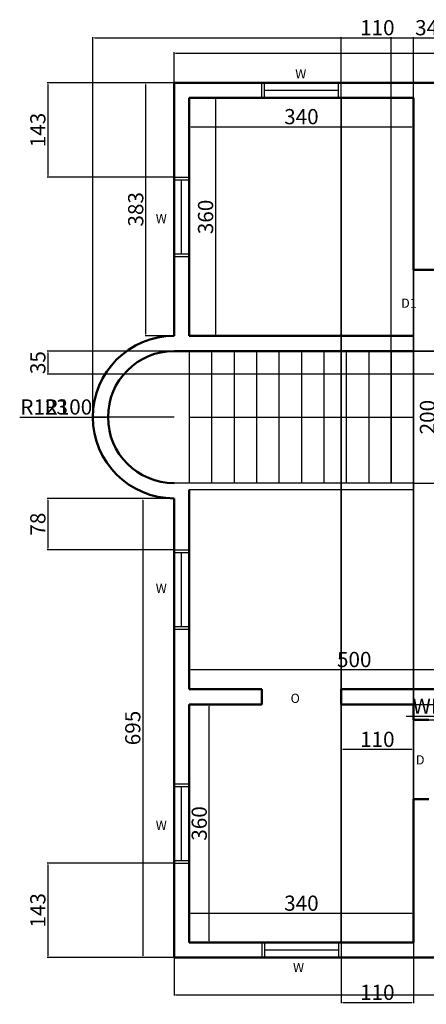
# Model space of a CAD drawing. Units: centimetres. Extents: x 6294 to 7898, y 3240 to 4730.
# Tile 1 of 3: x 6294 to 6910, y 3240 to 4730. Entities that reach past the tile are written whole.
import ezdxf

# ---------------------------------------------------------------- set-up
doc = ezdxf.new("R2010")
doc.units = ezdxf.units.CM
for name, color, linetype, lineweight in [('A-ANNO-DIMS', 2, 'Continuous', 18), ('A-ANNO-TEXT', 7, 'Continuous', 25), ('A-FLOR-STRS', 3, 'Continuous', 25), ('A-GLAZ', 4, 'Continuous', 25), ('A-WALL', 7, 'Continuous', 50)]:
    doc.layers.add(name, color=color, linetype=linetype, lineweight=lineweight)
doc.styles.get("Standard").update_dxf_attribs({"font": 'arial.ttf'})
doc.dimstyles.new('ISO-25', dxfattribs={"dimtxt": 23, "dimasz": 2.5, "dimexe": 1.25, "dimexo": 0.625, "dimtad": 1, "dimtxsty": 'Standard', "dimcen": 2.5, "dimadec": 0, "dimazin": 0, "dimtfac": 1, "dimtmove": 0, "dimatfit": 3, "dimfxl": 1, "dimarcsym": 0})

# ---------------------------------------------------------------- blocks, each defined once
blk = doc.blocks.new('*D2')
at = {"layer": 'A-ANNO-DIMS', "color": 0, "lineweight": -2, "transparency": 16777216}
for p, q in [((6551.4, 4611.8), (6592.1, 4611.8)), ((6590.8, 4254.3), (6590.8, 4609.3)), ((6551.4, 4251.8), (6592.1, 4251.8))]:
    blk.add_line(p, q, dxfattribs=at)
at = {"layer": 'A-ANNO-DIMS', "color": 0, "transparency": 16777216}
for points in [[(6590.4, 4609.3), (6591.3, 4609.3), (6590.8, 4611.8)], [(6590.4, 4254.3), (6591.3, 4254.3), (6590.8, 4251.8)]]:
    blk.add_solid(points, dxfattribs=at)
at = {"layer": 'Defpoints', "color": 0, "transparency": 16777216}
for p in [(6550.7, 4611.8), (6590.8, 4611.8), (6550.7, 4251.8)]:
    blk.add_point(p, dxfattribs=at)
at = {"layer": 'A-ANNO-DIMS', "color": 0, "transparency": 16777216, "insert": (6578.5, 4431.8), "char_height": 23, "attachment_point": 5, "rotation": 90}
blk.add_mtext('360', dxfattribs=at)
blk = doc.blocks.new('*D3')
at = {"layer": 'A-ANNO-DIMS', "color": 0, "lineweight": -2, "transparency": 16777216}
for p, q in [((6550.7, 4611.2), (6550.7, 4566.9)), ((6890.7, 4611.2), (6890.7, 4566.9)), ((6553.2, 4568.2), (6888.2, 4568.2))]:
    blk.add_line(p, q, dxfattribs=at)
at = {"layer": 'A-ANNO-DIMS', "color": 0, "transparency": 16777216}
for points in [[(6553.2, 4568.6), (6553.2, 4567.8), (6550.7, 4568.2)], [(6888.2, 4568.6), (6888.2, 4567.8), (6890.7, 4568.2)]]:
    blk.add_solid(points, dxfattribs=at)
at = {"layer": 'Defpoints', "color": 0, "transparency": 16777216}
for p in [(6550.7, 4611.8), (6890.7, 4611.8), (6890.7, 4568.2)]:
    blk.add_point(p, dxfattribs=at)
at = {"layer": 'A-ANNO-DIMS', "color": 0, "transparency": 16777216, "insert": (6720.7, 4580.6), "char_height": 23, "attachment_point": 5}
blk.add_mtext('340', dxfattribs=at)
blk = doc.blocks.new('*D18')
at = {"layer": 'A-ANNO-DIMS', "color": 0, "lineweight": -2, "transparency": 16777216}
for p, q in [((6551.4, 3693.8), (6582.5, 3693.8)), ((6581.2, 3336.3), (6581.2, 3691.3)), ((6551.4, 3333.8), (6582.5, 3333.8))]:
    blk.add_line(p, q, dxfattribs=at)
at = {"layer": 'A-ANNO-DIMS', "color": 0, "transparency": 16777216}
for points in [[(6580.8, 3691.3), (6581.7, 3691.3), (6581.2, 3693.8)], [(6580.8, 3336.3), (6581.7, 3336.3), (6581.2, 3333.8)]]:
    blk.add_solid(points, dxfattribs=at)
at = {"layer": 'Defpoints', "color": 0, "transparency": 16777216}
for p in [(6550.7, 3693.8), (6581.2, 3693.8), (6550.7, 3333.8)]:
    blk.add_point(p, dxfattribs=at)
at = {"layer": 'A-ANNO-DIMS', "color": 0, "transparency": 16777216, "insert": (6568.9, 3513.8), "char_height": 23, "attachment_point": 5, "rotation": 90}
blk.add_mtext('360', dxfattribs=at)
blk = doc.blocks.new('*D19')
at = {"layer": 'A-ANNO-DIMS', "color": 0, "lineweight": -2, "transparency": 16777216}
for p, q in [((6550.7, 3334.5), (6550.7, 3379.1)), ((6553.2, 3377.9), (6888.2, 3377.9)), ((6890.7, 3334.5), (6890.7, 3379.1))]:
    blk.add_line(p, q, dxfattribs=at)
at = {"layer": 'A-ANNO-DIMS', "color": 0, "transparency": 16777216}
for points in [[(6553.2, 3378.3), (6553.2, 3377.4), (6550.7, 3377.9)], [(6888.2, 3378.3), (6888.2, 3377.4), (6890.7, 3377.9)]]:
    blk.add_solid(points, dxfattribs=at)
at = {"layer": 'Defpoints', "color": 0, "transparency": 16777216}
for p in [(6890.7, 3377.9), (6550.7, 3333.8), (6890.7, 3333.8)]:
    blk.add_point(p, dxfattribs=at)
at = {"layer": 'A-ANNO-DIMS', "color": 0, "transparency": 16777216, "insert": (6720.7, 3390.2), "char_height": 23, "attachment_point": 5}
blk.add_mtext('340', dxfattribs=at)
blk = doc.blocks.new('*D20')
at = {"layer": 'A-ANNO-DIMS', "color": 0, "lineweight": -2, "transparency": 16777216}
for p, q in [((6550.7, 3717.5), (6550.7, 3747.9)), ((6553.2, 3746.6), (7048.2, 3746.6)), ((7050.7, 3717.5), (7050.7, 3747.9))]:
    blk.add_line(p, q, dxfattribs=at)
at = {"layer": 'A-ANNO-DIMS', "color": 0, "transparency": 16777216}
for points in [[(6553.2, 3747), (6553.2, 3746.2), (6550.7, 3746.6)], [(7048.2, 3747), (7048.2, 3746.2), (7050.7, 3746.6)]]:
    blk.add_solid(points, dxfattribs=at)
at = {"layer": 'Defpoints', "color": 0, "transparency": 16777216}
for p in [(7050.7, 3746.6), (6550.7, 3716.8), (7050.7, 3716.8)]:
    blk.add_point(p, dxfattribs=at)
at = {"layer": 'A-ANNO-DIMS', "color": 0, "transparency": 16777216, "insert": (6800.7, 3759), "char_height": 23, "attachment_point": 5}
blk.add_mtext('500', dxfattribs=at)
blk = doc.blocks.new('*D22')
at = {"layer": 'A-ANNO-DIMS', "color": 0, "lineweight": -2, "transparency": 16777216}
for p, q in [((6891.4, 4228.8), (6928.2, 4228.8)), ((6926.9, 4226.3), (6926.9, 4031.3)), ((6891.4, 4028.8), (6928.2, 4028.8))]:
    blk.add_line(p, q, dxfattribs=at)
at = {"layer": 'A-ANNO-DIMS', "color": 0, "transparency": 16777216}
for points in [[(6926.5, 4226.3), (6927.3, 4226.3), (6926.9, 4228.8)], [(6926.5, 4031.3), (6927.3, 4031.3), (6926.9, 4028.8)]]:
    blk.add_solid(points, dxfattribs=at)
at = {"layer": 'Defpoints', "color": 0, "transparency": 16777216}
for p in [(6890.7, 4228.8), (6890.7, 4028.8), (6926.9, 4028.8)]:
    blk.add_point(p, dxfattribs=at)
at = {"layer": 'A-ANNO-DIMS', "color": 0, "transparency": 16777216, "insert": (6914.6, 4128.8), "char_height": 23, "attachment_point": 5, "rotation": 90}
blk.add_mtext('200', dxfattribs=at)
blk = doc.blocks.new('*D23')
at = {"layer": 'A-ANNO-DIMS', "color": 0, "lineweight": -2, "transparency": 16777216}
for p, q in [((6527.7, 4635.5), (6527.7, 4681.1)), ((6530.2, 4679.8), (7596.2, 4679.8)), ((7598.7, 4635.5), (7598.7, 4681.1))]:
    blk.add_line(p, q, dxfattribs=at)
at = {"layer": 'A-ANNO-DIMS', "color": 0, "transparency": 16777216}
for points in [[(6530.2, 4680.2), (6530.2, 4679.4), (6527.7, 4679.8)], [(7596.2, 4680.2), (7596.2, 4679.4), (7598.7, 4679.8)]]:
    blk.add_solid(points, dxfattribs=at)
at = {"layer": 'Defpoints', "color": 0, "transparency": 16777216}
for p in [(7598.7, 4679.8), (6527.7, 4634.8), (7598.7, 4634.8)]:
    blk.add_point(p, dxfattribs=at)
at = {"layer": 'A-ANNO-DIMS', "color": 0, "transparency": 16777216, "insert": (7063.2, 4692.2), "char_height": 23, "attachment_point": 5}
blk.add_mtext('1071', dxfattribs=at)
blk = doc.blocks.new('*D26')
at = {"layer": 'A-ANNO-DIMS', "color": 0, "lineweight": -2, "transparency": 16777216}
for p, q in [((6527.7, 3310.2), (6527.7, 3253.3)), ((7396.7, 3310.2), (7396.7, 3253.3)), ((6530.2, 3254.6), (7394.2, 3254.6))]:
    blk.add_line(p, q, dxfattribs=at)
at = {"layer": 'A-ANNO-DIMS', "color": 0, "transparency": 16777216}
for points in [[(6530.2, 3255), (6530.2, 3254.2), (6527.7, 3254.6)], [(7394.2, 3255), (7394.2, 3254.2), (7396.7, 3254.6)]]:
    blk.add_solid(points, dxfattribs=at)
at = {"layer": 'Defpoints', "color": 0, "transparency": 16777216}
for p in [(6527.7, 3310.8), (7396.7, 3310.8), (7396.7, 3254.6)]:
    blk.add_point(p, dxfattribs=at)
at = {"layer": 'A-ANNO-DIMS', "color": 0, "transparency": 16777216, "insert": (6962.2, 3266.9), "char_height": 23, "attachment_point": 5}
blk.add_mtext('869', dxfattribs=at)
blk = doc.blocks.new('*D27')
at = {"layer": 'A-ANNO-DIMS', "color": 0, "lineweight": -2, "transparency": 16777216}
for p, q in [((6527.1, 4005.8), (6479.3, 4005.8)), ((6480.6, 4003.3), (6480.6, 3313.3)), ((6527.1, 3310.8), (6479.3, 3310.8))]:
    blk.add_line(p, q, dxfattribs=at)
at = {"layer": 'A-ANNO-DIMS', "color": 0, "transparency": 16777216}
for points in [[(6480.2, 4003.3), (6481, 4003.3), (6480.6, 4005.8)], [(6480.2, 3313.3), (6481, 3313.3), (6480.6, 3310.8)]]:
    blk.add_solid(points, dxfattribs=at)
at = {"layer": 'Defpoints', "color": 0, "transparency": 16777216}
for p in [(6527.7, 4005.8), (6480.6, 3310.8), (6527.7, 3310.8)]:
    blk.add_point(p, dxfattribs=at)
at = {"layer": 'A-ANNO-DIMS', "color": 0, "transparency": 16777216, "insert": (6468.2, 3658.3), "char_height": 23, "attachment_point": 5, "rotation": 90}
blk.add_mtext('695', dxfattribs=at)
blk = doc.blocks.new('*D28')
at = {"layer": 'A-ANNO-DIMS', "color": 0, "lineweight": -2, "transparency": 16777216}
for p, q in [((6527.1, 4634.8), (6483.8, 4634.8)), ((6485.1, 4254.3), (6485.1, 4632.3)), ((6527.1, 4251.8), (6483.8, 4251.8))]:
    blk.add_line(p, q, dxfattribs=at)
at = {"layer": 'A-ANNO-DIMS', "color": 0, "transparency": 16777216}
for points in [[(6484.7, 4632.3), (6485.5, 4632.3), (6485.1, 4634.8)], [(6484.7, 4254.3), (6485.5, 4254.3), (6485.1, 4251.8)]]:
    blk.add_solid(points, dxfattribs=at)
at = {"layer": 'Defpoints', "color": 0, "transparency": 16777216}
for p in [(6485.1, 4634.8), (6527.7, 4634.8), (6527.7, 4251.8)]:
    blk.add_point(p, dxfattribs=at)
at = {"layer": 'A-ANNO-DIMS', "color": 0, "transparency": 16777216, "insert": (6472.7, 4443.3), "char_height": 23, "attachment_point": 5, "rotation": 90}
blk.add_mtext('383', dxfattribs=at)
blk = doc.blocks.new('WIN-W-120CM')
for p, q in [((0, 23), (0, 0)), ((4, 23), (4, 0)), ((116, 23), (116, 0)), ((120, 23), (120, 0)), ((4, 11.5), (116, 11.5))]:
    blk.add_line(p, q)
blk = doc.blocks.new('*D32')
at = {"layer": 'A-ANNO-DIMS', "color": 0, "lineweight": -2, "transparency": 16777216}
for p, q in [((7163.7, 3693.2), (7163.7, 3674.6)), ((7283.7, 3693.2), (7283.7, 3674.6)), ((7163.7, 3675.8), (6879.3, 3675.8)), ((7281.2, 3675.8), (7166.2, 3675.8))]:
    blk.add_line(p, q, dxfattribs=at)
at = {"layer": 'A-ANNO-DIMS', "color": 0, "transparency": 16777216}
for points in [[(7166.2, 3676.3), (7166.2, 3675.4), (7163.7, 3675.8)], [(7281.2, 3676.3), (7281.2, 3675.4), (7283.7, 3675.8)]]:
    blk.add_solid(points, dxfattribs=at)
at = {"layer": 'Defpoints', "color": 0, "transparency": 16777216}
for p in [(7163.7, 3693.8), (7283.7, 3693.8), (7163.7, 3675.8)]:
    blk.add_point(p, dxfattribs=at)
at = {"layer": 'A-ANNO-DIMS', "color": 0, "transparency": 16777216, "insert": (7020.3, 3688.4), "char_height": 23, "attachment_point": 5}
blk.add_mtext('WINDOW 120 TYP.', dxfattribs=at)
blk = doc.blocks.new('*D39')
at = {"layer": 'A-ANNO-DIMS', "color": 0, "lineweight": -2, "transparency": 16777216}
for p, q in [((6404.7, 4129.5), (6404.7, 4704.1)), ((6407.2, 4702.8), (7596.2, 4702.8)), ((7598.7, 4635.5), (7598.7, 4704.1))]:
    blk.add_line(p, q, dxfattribs=at)
at = {"layer": 'A-ANNO-DIMS', "color": 0, "transparency": 16777216}
for points in [[(6407.2, 4703.3), (6407.2, 4702.4), (6404.7, 4702.8)], [(7596.2, 4703.3), (7596.2, 4702.4), (7598.7, 4702.8)]]:
    blk.add_solid(points, dxfattribs=at)
at = {"layer": 'Defpoints', "color": 0, "transparency": 16777216}
for p in [(7598.7, 4702.8), (7598.7, 4634.8), (6404.7, 4128.8)]:
    blk.add_point(p, dxfattribs=at)
at = {"layer": 'A-ANNO-DIMS', "color": 0, "transparency": 16777216, "insert": (7001.7, 4715.2), "char_height": 23, "attachment_point": 5}
blk.add_mtext('1194', dxfattribs=at)
blk = doc.blocks.new('*D40')
at = {"layer": 'A-ANNO-DIMS', "color": 0, "lineweight": -2, "transparency": 16777216}
for p, q in [((6856.7, 4029.5), (6856.7, 4704.1)), ((6859.2, 4702.8), (6888.2, 4702.8)), ((6890.7, 4029.5), (6890.7, 4704.1)), ((6890.7, 4702.8), (6927.3, 4702.8))]:
    blk.add_line(p, q, dxfattribs=at)
at = {"layer": 'A-ANNO-DIMS', "color": 0, "transparency": 16777216}
for points in [[(6859.2, 4703.3), (6859.2, 4702.4), (6856.7, 4702.8)], [(6888.2, 4703.3), (6888.2, 4702.4), (6890.7, 4702.8)]]:
    blk.add_solid(points, dxfattribs=at)
at = {"layer": 'Defpoints', "color": 0, "transparency": 16777216}
for p in [(6890.7, 4702.8), (6856.7, 4028.8), (6890.7, 4028.8)]:
    blk.add_point(p, dxfattribs=at)
at = {"layer": 'A-ANNO-DIMS', "color": 0, "transparency": 16777216, "insert": (6910.3, 4715.2), "char_height": 23, "attachment_point": 5}
blk.add_mtext('34', dxfattribs=at)
blk = doc.blocks.new('*D41')
at = {"layer": 'A-ANNO-DIMS', "color": 0, "lineweight": -2, "transparency": 16777216}
for p, q in [((6527.1, 4005.8), (6335.5, 4005.8)), ((6336.7, 4003.3), (6336.7, 3930.3)), ((6527.1, 3927.8), (6335.5, 3927.8))]:
    blk.add_line(p, q, dxfattribs=at)
at = {"layer": 'A-ANNO-DIMS', "color": 0, "transparency": 16777216}
for points in [[(6336.3, 4003.3), (6337.2, 4003.3), (6336.7, 4005.8)], [(6336.3, 3930.3), (6337.2, 3930.3), (6336.7, 3927.8)]]:
    blk.add_solid(points, dxfattribs=at)
at = {"layer": 'Defpoints', "color": 0, "transparency": 16777216}
for p in [(6527.7, 4005.8), (6336.7, 3927.8), (6527.7, 3927.8)]:
    blk.add_point(p, dxfattribs=at)
at = {"layer": 'A-ANNO-DIMS', "color": 0, "transparency": 16777216, "insert": (6324.4, 3966.8), "char_height": 23, "attachment_point": 5, "rotation": 90}
blk.add_mtext('78', dxfattribs=at)
blk = doc.blocks.new('*D42')
at = {"layer": 'A-ANNO-DIMS', "color": 0, "lineweight": -2, "transparency": 16777216}
for p, q in [((6780.7, 3334.5), (6780.7, 4704.1)), ((6783.2, 4702.8), (6888.2, 4702.8)), ((6890.7, 3334.5), (6890.7, 4704.1))]:
    blk.add_line(p, q, dxfattribs=at)
at = {"layer": 'A-ANNO-DIMS', "color": 0, "transparency": 16777216}
for points in [[(6783.2, 4703.3), (6783.2, 4702.4), (6780.7, 4702.8)], [(6888.2, 4703.3), (6888.2, 4702.4), (6890.7, 4702.8)]]:
    blk.add_solid(points, dxfattribs=at)
at = {"layer": 'Defpoints', "color": 0, "transparency": 16777216}
for p in [(6890.7, 4702.8), (6780.7, 3333.8), (6890.7, 3333.8)]:
    blk.add_point(p, dxfattribs=at)
at = {"layer": 'A-ANNO-DIMS', "color": 0, "transparency": 16777216, "insert": (6835.7, 4715.2), "char_height": 23, "attachment_point": 5}
blk.add_mtext('110', dxfattribs=at)
blk = doc.blocks.new('*D43')
at = {"layer": 'A-ANNO-DIMS', "color": 0, "lineweight": -2, "transparency": 16777216}
for p, q in [((6527.1, 3453.8), (6335.5, 3453.8)), ((6336.7, 3451.3), (6336.7, 3313.3)), ((6527.1, 3310.8), (6335.5, 3310.8))]:
    blk.add_line(p, q, dxfattribs=at)
at = {"layer": 'A-ANNO-DIMS', "color": 0, "transparency": 16777216}
for points in [[(6336.3, 3451.3), (6337.2, 3451.3), (6336.7, 3453.8)], [(6336.3, 3313.3), (6337.2, 3313.3), (6336.7, 3310.8)]]:
    blk.add_solid(points, dxfattribs=at)
at = {"layer": 'Defpoints', "color": 0, "transparency": 16777216}
for p in [(6527.7, 3453.8), (6336.7, 3310.8), (6527.7, 3310.8)]:
    blk.add_point(p, dxfattribs=at)
at = {"layer": 'A-ANNO-DIMS', "color": 0, "transparency": 16777216, "insert": (6324.4, 3382.3), "char_height": 23, "attachment_point": 5, "rotation": 90}
blk.add_mtext('143', dxfattribs=at)
blk = doc.blocks.new('*D44')
at = {"layer": 'A-ANNO-DIMS', "color": 0, "lineweight": -2, "transparency": 16777216}
for p, q in [((6891.4, 3693.8), (7668, 3693.8)), ((7666.7, 3691.3), (7666.7, 3673.3)), ((6891.4, 3670.8), (7668, 3670.8)), ((7666.7, 3670.8), (7666.7, 3633.8))]:
    blk.add_line(p, q, dxfattribs=at)
at = {"layer": 'A-ANNO-DIMS', "color": 0, "transparency": 16777216}
for points in [[(7666.3, 3691.3), (7667.2, 3691.3), (7666.7, 3693.8)], [(7666.3, 3673.3), (7667.2, 3673.3), (7666.7, 3670.8)]]:
    blk.add_solid(points, dxfattribs=at)
at = {"layer": 'Defpoints', "color": 0, "transparency": 16777216}
for p in [(6890.7, 3693.8), (6890.7, 3670.8), (7666.7, 3670.8)]:
    blk.add_point(p, dxfattribs=at)
at = {"layer": 'A-ANNO-DIMS', "color": 0, "transparency": 16777216, "insert": (7654.4, 3651.1), "char_height": 23, "attachment_point": 5, "rotation": 90}
blk.add_mtext('23', dxfattribs=at)
blk = doc.blocks.new('*D45')
at = {"layer": 'A-ANNO-DIMS', "color": 0, "lineweight": -2, "transparency": 16777216}
for p, q in [((6780.7, 4611.2), (6780.7, 3241.6)), ((6890.7, 4611.2), (6890.7, 3241.6)), ((6783.2, 3242.8), (6888.2, 3242.8))]:
    blk.add_line(p, q, dxfattribs=at)
at = {"layer": 'A-ANNO-DIMS', "color": 0, "transparency": 16777216}
for points in [[(6783.2, 3243.3), (6783.2, 3242.4), (6780.7, 3242.8)], [(6888.2, 3243.3), (6888.2, 3242.4), (6890.7, 3242.8)]]:
    blk.add_solid(points, dxfattribs=at)
at = {"layer": 'Defpoints', "color": 0, "transparency": 16777216}
for p in [(6780.7, 4611.8), (6890.7, 4611.8), (6890.7, 3242.8)]:
    blk.add_point(p, dxfattribs=at)
at = {"layer": 'A-ANNO-DIMS', "color": 0, "transparency": 16777216, "insert": (6835.7, 3255.2), "char_height": 23, "attachment_point": 5}
blk.add_mtext('110', dxfattribs=at)
blk = doc.blocks.new('*D48')
at = {"layer": 'A-ANNO-DIMS', "color": 0, "lineweight": -2, "transparency": 16777216}
for p, q in [((6527.1, 4634.8), (6335.5, 4634.8)), ((6336.7, 4632.3), (6336.7, 4494.3)), ((6527.1, 4491.8), (6335.5, 4491.8))]:
    blk.add_line(p, q, dxfattribs=at)
at = {"layer": 'A-ANNO-DIMS', "color": 0, "transparency": 16777216}
for points in [[(6336.3, 4632.3), (6337.2, 4632.3), (6336.7, 4634.8)], [(6336.3, 4494.3), (6337.2, 4494.3), (6336.7, 4491.8)]]:
    blk.add_solid(points, dxfattribs=at)
at = {"layer": 'Defpoints', "color": 0, "transparency": 16777216}
for p in [(6527.7, 4634.8), (6336.7, 4491.8), (6527.7, 4491.8)]:
    blk.add_point(p, dxfattribs=at)
at = {"layer": 'A-ANNO-DIMS', "color": 0, "transparency": 16777216, "insert": (6324.4, 4563.3), "char_height": 23, "attachment_point": 5, "rotation": 90}
blk.add_mtext('143', dxfattribs=at)
blk = doc.blocks.new('*D49')
at = {"layer": 'A-ANNO-DIMS', "color": 0, "lineweight": -2, "transparency": 16777216}
for p, q in [((7373.1, 4228.8), (6335.5, 4228.8)), ((6336.7, 4226.3), (6336.7, 4196.3)), ((7373.1, 4193.8), (6335.5, 4193.8))]:
    blk.add_line(p, q, dxfattribs=at)
at = {"layer": 'A-ANNO-DIMS', "color": 0, "transparency": 16777216}
for points in [[(6336.3, 4226.3), (6337.2, 4226.3), (6336.7, 4228.8)], [(6336.3, 4196.3), (6337.2, 4196.3), (6336.7, 4193.8)]]:
    blk.add_solid(points, dxfattribs=at)
at = {"layer": 'Defpoints', "color": 0, "transparency": 16777216}
for p in [(7373.7, 4228.8), (6336.7, 4193.8), (7373.7, 4193.8)]:
    blk.add_point(p, dxfattribs=at)
at = {"layer": 'A-ANNO-DIMS', "color": 0, "transparency": 16777216, "insert": (6324.4, 4211.3), "char_height": 23, "attachment_point": 5, "rotation": 90}
blk.add_mtext('35', dxfattribs=at)
blk = doc.blocks.new('*D52')
at = {"layer": 'A-ANNO-DIMS', "color": 0, "lineweight": -2, "transparency": 16777216}
for p, q in [((6780.7, 3693.2), (6780.7, 3624.6)), ((6890.7, 3693.2), (6890.7, 3624.6)), ((6888.2, 3625.8), (6783.2, 3625.8))]:
    blk.add_line(p, q, dxfattribs=at)
at = {"layer": 'A-ANNO-DIMS', "color": 0, "transparency": 16777216}
for points in [[(6783.2, 3626.3), (6783.2, 3625.4), (6780.7, 3625.8)], [(6888.2, 3626.3), (6888.2, 3625.4), (6890.7, 3625.8)]]:
    blk.add_solid(points, dxfattribs=at)
at = {"layer": 'Defpoints', "color": 0, "transparency": 16777216}
for p in [(6780.7, 3693.8), (6890.7, 3693.8), (6780.7, 3625.8)]:
    blk.add_point(p, dxfattribs=at)
at = {"layer": 'A-ANNO-DIMS', "color": 0, "transparency": 16777216, "insert": (6835.7, 3638.2), "char_height": 23, "attachment_point": 5}
blk.add_mtext('110', dxfattribs=at)
blk = doc.blocks.new('*D54')
at = {"layer": 'A-ANNO-DIMS', "color": 0, "lineweight": -2, "transparency": 16777216}
for p, q in [((6293.9, 4128.8), (6402.2, 4128.8)), ((6527.7, 4128.8), (6404.7, 4128.8))]:
    blk.add_line(p, q, dxfattribs=at)
at = {"layer": 'A-ANNO-DIMS', "color": 0, "transparency": 16777216}
blk.add_solid([(6402.2, 4129.3), (6402.2, 4128.4), (6404.7, 4128.8)], dxfattribs=at)
at = {"layer": 'Defpoints', "color": 0, "transparency": 16777216}
for p in [(6404.7, 4128.8), (6527.7, 4128.8)]:
    blk.add_point(p, dxfattribs=at)
at = {"layer": 'A-ANNO-DIMS', "color": 0, "transparency": 16777216, "insert": (6330.9, 4141.2), "char_height": 23, "attachment_point": 5}
blk.add_mtext('R123', dxfattribs=at)
blk = doc.blocks.new('*D55')
at = {"layer": 'A-ANNO-DIMS', "color": 0, "lineweight": -2, "transparency": 16777216}
for p, q in [((6330.7, 4128.8), (6425.2, 4128.8)), ((6527.7, 4128.8), (6427.7, 4128.8))]:
    blk.add_line(p, q, dxfattribs=at)
at = {"layer": 'A-ANNO-DIMS', "color": 0, "transparency": 16777216}
blk.add_solid([(6425.2, 4129.3), (6425.2, 4128.4), (6427.7, 4128.8)], dxfattribs=at)
at = {"layer": 'Defpoints', "color": 0, "transparency": 16777216}
for p in [(6427.7, 4128.8), (6527.7, 4128.8)]:
    blk.add_point(p, dxfattribs=at)
at = {"layer": 'A-ANNO-DIMS', "color": 0, "transparency": 16777216, "insert": (6367.7, 4141.2), "char_height": 23, "attachment_point": 5}
blk.add_mtext('R100', dxfattribs=at)

msp = doc.modelspace()

# ---------------------------------------------------------------- linework, layer by layer
at = {"layer": 'A-FLOR-STRS'}
for p, q in [((6890.735, 4251.848), (6890.735, 4018.848)), ((6550.735, 4228.848), (6550.735, 4028.848)), ((6584.735, 4228.848), (6584.735, 4028.848)), ((6618.735, 4228.848), (6618.735, 4028.848)), ((6652.735, 4228.848), (6652.735, 4028.848)), ((6686.735, 4228.848), (6686.735, 4028.848)), ((6720.735, 4228.848), (6720.735, 4028.848)), ((6754.735, 4228.848), (6754.735, 4028.848)), ((6788.735, 4228.848), (6788.735, 4028.848)), ((6822.735, 4228.848), (6822.735, 4028.848)), ((6856.735, 4228.848), (6856.735, 4028.848)), ((6550.735, 4128.848), (6890.735, 4128.848)), ((6890.735, 4028.848), (6527.735, 4028.848)), ((6890.735, 4018.848), (6550.735, 4018.848))]:
    msp.add_line(p, q, dxfattribs=at)
at = {"layer": 'A-WALL'}
for p, q in [((7598.735, 4634.848), (6527.735, 4634.848)), ((6527.735, 4634.848), (6527.735, 4251.848)), ((6550.735, 4611.848), (6550.735, 4251.848)), ((6890.735, 4611.848), (6550.735, 4611.848)), ((6890.735, 4611.848), (6890.735, 4351.848)), ((7083.735, 4351.848), (6890.735, 4351.848)), ((6890.735, 4251.848), (6550.735, 4251.848)), ((6890.735, 4228.848), (6527.735, 4228.848)), ((6550.735, 4018.848), (6550.735, 3716.848)), ((6527.735, 4005.848), (6527.735, 3310.848)), ((6660.735, 3716.848), (6550.735, 3716.848)), ((6660.735, 3693.848), (6660.735, 3716.848)), ((7050.735, 3716.848), (6780.735, 3716.848)), ((6780.735, 3693.848), (6780.735, 3716.848)), ((6550.735, 3693.848), (6550.735, 3333.848)), ((6660.735, 3693.848), (6550.735, 3693.848)), ((6890.735, 3693.848), (6780.735, 3693.848)), ((6890.735, 3693.848), (6890.735, 3670.848)), ((6913.735, 3670.848), (6890.735, 3670.848)), ((6890.735, 3550.848), (6890.735, 3333.848)), ((6913.735, 3550.848), (6890.735, 3550.848)), ((6890.735, 3333.848), (6550.735, 3333.848)), ((7396.735, 3310.848), (6527.735, 3310.848))]:
    msp.add_line(p, q, dxfattribs=at)
for radius in [123, 100]:
    msp.add_arc((6527.735, 4128.848), radius, 90, 270, dxfattribs=at)

# ---------------------------------------------------------------- block references
at = {"layer": 'A-GLAZ'}
for p, rotation in [((6780.735, 4634.848), 180), ((6550.735, 4371.848), 90.00000000000067), ((6550.735, 3807.848), 90.00000000000063), ((6550.735, 3453.848), 90.0000000000016)]:
    msp.add_blockref('WIN-W-120CM', p, dxfattribs=dict(at, rotation=rotation))
msp.add_blockref('WIN-W-120CM', (6660.735, 3310.848), dxfattribs=at)

# ---------------------------------------------------------------- texts
at = {"layer": 'A-ANNO-TEXT'}
for s, height, p in [('W', 13.978, (6711.334, 4641.332)), ('W', 13.978, (6500.024, 4422.35)), ('D1', 13.9778, (6871.715, 4294.279)), ('W', 13.978, (6500.024, 3862.645)), ('O ', 13.9778, (6704.26, 3696.204)), ('D', 13.978, (6894.112, 3603.117)), ('W', 13.978, (6500.024, 3504.008)), ('W', 13.978, (6707.973, 3288.804))]:
    msp.add_text(s, height=height, dxfattribs=at).set_placement(p)

# ---------------------------------------------------------------- dimensions: what is measured, and where the dimension line sits
at = {"layer": 'A-ANNO-DIMS'}
for base, p1, p2, override, picture, middle in [((7598.735, 4702.848), (6404.735, 4128.848), (7598.735, 4634.848), {"dimdec": 0, "dimlfac": 1, "dimrnd": 0, "dimzin": 0, "dimdsep": 46, "dimlunit": 2}, '*D39', (7001.735, 4715.216)), ((6890.735, 4702.848), (6780.735, 3333.848), (6890.735, 3333.848), {"dimdec": 0, "dimlfac": 1, "dimrnd": 0, "dimzin": 0, "dimdsep": 46, "dimlunit": 2}, '*D42', (6835.735, 4715.216)), ((6890.735, 4702.848), (6856.735, 4028.848), (6890.735, 4028.848), {"dimdec": 0, "dimlfac": 1, "dimrnd": 0, "dimzin": 0, "dimdsep": 46, "dimlunit": 2}, '*D40', (6910.278, 4715.224)), ((7598.735, 4679.801), (6527.735, 4634.848), (7598.735, 4634.848), {"dimclrd": 0, "dimclre": 0, "dimclrt": 0}, '*D23', (7063.235, 4692.17)), ((6890.735, 4568.181), (6550.735, 4611.848), (6890.735, 4611.848), {"dimclrd": 0, "dimclre": 0, "dimclrt": 0}, '*D3', (6720.735, 4580.557)), ((6890.735, 3242.848), (6780.735, 4611.848), (6890.735, 4611.848), {"dimdec": 0, "dimlfac": 1, "dimrnd": 0, "dimzin": 0, "dimdsep": 46, "dimlunit": 2}, '*D45', (6835.735, 3255.216)), ((7050.735, 3746.629), (6550.735, 3716.848), (7050.735, 3716.848), {"dimclrd": 0, "dimclre": 0, "dimclrt": 0}, '*D20', (6800.735, 3758.997)), ((6890.735, 3377.855), (6550.735, 3333.848), (6890.735, 3333.848), {"dimclrd": 0, "dimclre": 0, "dimclrt": 0}, '*D19', (6720.735, 3390.231)), ((7396.735, 3254.57), (6527.735, 3310.848), (7396.735, 3310.848), {"dimclrd": 0, "dimclre": 0, "dimclrt": 0}, '*D26', (6962.235, 3266.938))]:
    dim = msp.add_linear_dim(base=base, p1=p1, p2=p2, dimstyle='ISO-25', override=override, dxfattribs=at)
    dim.commit()
    dim.dimension.update_dxf_attribs({"geometry": picture, "text_midpoint": middle})
for base, p1, p2, angle, override, picture, middle in [((6336.735, 4491.848), (6527.735, 4634.848), (6527.735, 4491.848), 90, {"dimdec": 0, "dimlfac": 1, "dimrnd": 0, "dimzin": 0, "dimdsep": 46, "dimlunit": 2}, '*D48', (6324.359, 4563.348)), ((6485.097, 4634.848), (6527.735, 4251.848), (6527.735, 4634.848), 90, {"dimclrd": 0, "dimclre": 0, "dimclrt": 0}, '*D28', (6472.721, 4443.348)), ((6590.834, 4611.848), (6550.735, 4251.848), (6550.735, 4611.848), 270, {"dimclrd": 0, "dimclre": 0, "dimclrt": 0}, '*D2', (6578.458, 4431.848)), ((6336.735, 4193.848), (7373.735, 4228.848), (7373.735, 4193.848), 90, {"dimdec": 0, "dimlfac": 1, "dimrnd": 0, "dimzin": 0, "dimdsep": 46, "dimlunit": 2}, '*D49', (6324.359, 4211.348)), ((6926.928, 4028.848), (6890.735, 4228.848), (6890.735, 4028.848), 90, {"dimclrd": 0, "dimclre": 0, "dimclrt": 0}, '*D22', (6914.56, 4128.848)), ((6336.735, 3927.848), (6527.735, 4005.848), (6527.735, 3927.848), 90, {"dimdec": 0, "dimlfac": 1, "dimrnd": 0, "dimzin": 0, "dimdsep": 46, "dimlunit": 2}, '*D41', (6324.366, 3966.848)), ((6480.593, 3310.848), (6527.735, 4005.848), (6527.735, 3310.848), 90, {"dimclrd": 0, "dimclre": 0, "dimclrt": 0}, '*D27', (6468.225, 3658.348)), ((6581.236, 3693.848), (6550.735, 3333.848), (6550.735, 3693.848), 270, {"dimclrd": 0, "dimclre": 0, "dimclrt": 0}, '*D18', (6568.86, 3513.848)), ((6780.735, 3625.848), (6890.735, 3693.848), (6780.735, 3693.848), 180, {"dimdec": 0, "dimlfac": 1, "dimrnd": 0, "dimzin": 0, "dimdsep": 46, "dimlunit": 2}, '*D52', (6835.735, 3638.216)), ((7666.735, 3670.848), (6890.735, 3693.848), (6890.735, 3670.848), 90, {"dimdec": 0, "dimlfac": 1, "dimrnd": 0, "dimzin": 0, "dimdsep": 46, "dimlunit": 2}, '*D44', (7654.359, 3651.054)), ((6336.735, 3310.848), (6527.735, 3453.848), (6527.735, 3310.848), 90, {"dimdec": 0, "dimlfac": 1, "dimrnd": 0, "dimzin": 0, "dimdsep": 46, "dimlunit": 2}, '*D43', (6324.359, 3382.348))]:
    dim = msp.add_linear_dim(base=base, p1=p1, p2=p2, angle=angle, dimstyle='ISO-25', override=override, dxfattribs=at)
    dim.commit()
    dim.dimension.update_dxf_attribs({"geometry": picture, "text_midpoint": middle})
for mpoint, picture, middle in [((6404.735, 4128.848), '*D54', (6330.935, 4128.848)), ((6427.735, 4128.848), '*D55', (6367.735, 4128.848))]:
    dim = msp.add_radius_dim(center=(6527.735, 4128.848), mpoint=mpoint, dimstyle='ISO-25', override={"dimdec": 0, "dimlfac": 1, "dimrnd": 0, "dimzin": 0, "dimdsep": 46, "dimlunit": 2}, dxfattribs=at)
    dim.commit()
    dim.dimension.update_dxf_attribs({"geometry": picture, "text_midpoint": middle, "dimtype": 164})
dim = msp.add_linear_dim(base=(7163.735, 3675.848), p1=(7283.735, 3693.848), p2=(7163.735, 3693.848), angle=180, text='WINDOW <> TYP.', dimstyle='ISO-25', override={"dimdec": 0, "dimlfac": 1, "dimrnd": 0, "dimzin": 0, "dimdsep": 46, "dimlunit": 2}, dxfattribs=at)
dim.commit()
dim.dimension.update_dxf_attribs({"geometry": '*D32', "text_midpoint": (7020.272, 3688.373)})

doc.saveas('drawing.dxf')
